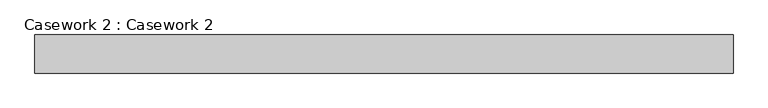
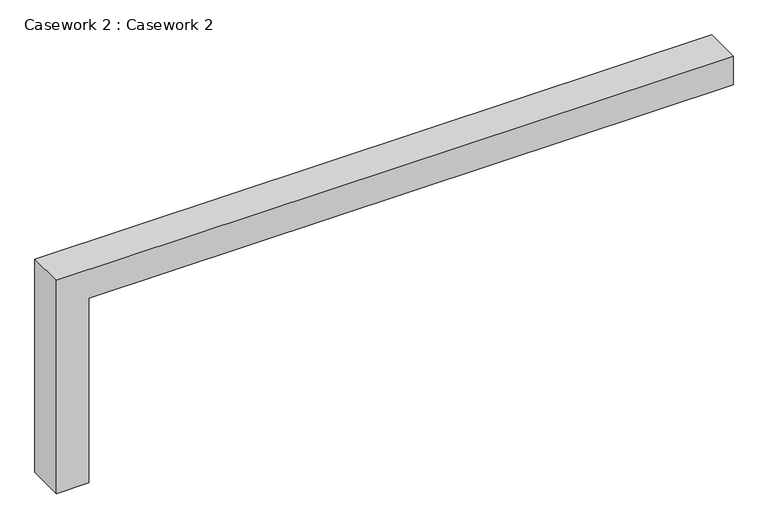
"""IFC4 building model written with IfcOpenShell, lengths in millimetres: furniture geometry, Casework 2 : Casework 2."""

from ifc_helpers import new_model, si_unit, frame, origin, place, context, project, spatial, polyline, outline, extrude, source, transform, mapped, element, save


def casework_2_casework_2_4a4ec244(model_context):
    return source(origin(), model_context, "Body", "SweptSolid", [
        extrude(outline(polyline([(5105.4, -20499.6994093), (-152.4, -20499.6994093), (-152.4, -19737.6994093), (4394.2, -19737.6994093), (4394.2, -4726.2994093), (5105.4, -4726.2994093), (5105.4, -20499.6994093)])), frame((0.0, -473.7110703, 0.0), z_axis=(0.0, 1.0, 0.0), x_axis=(0.0, 0.0, 1.0)), (0.0, 0.0, 1.0), 861.234819),
    ])


if __name__ == "__main__":
    model = new_model("IFC4")
    model_context = context("Model", 3, world=origin())
    ifc_project = project(units=[si_unit("LENGTHUNIT", "METRE", prefix="MILLI")], contexts=[model_context])
    site = spatial("IfcSite", under=ifc_project)
    building = spatial("IfcBuilding", under=site)
    placement = place(None, origin())
    casework_2_casework_2_shape = casework_2_casework_2_4a4ec244(model_context)
    element("IfcFurniture", 1, ObjectType="Casework 2 : Casework 2", at=placement, inside=building, context=model_context, shape_type="MappedRepresentation", body=[
        mapped(casework_2_casework_2_shape, transform((0.0, 0.0, 0.0), x_axis=(1.0, 0.0, 0.0), y_axis=(0.0, 1.0, 0.0), z_axis=(0.0, 0.0, 1.0))),
    ])
    save(model, "model.ifc")

# Revit data of these elements
# Element 1 (IfcFurniture, "Casework 2 : Casework 2")
#   Materials on its faces: "Clad - White"
# Materials
#   "Clad - White": class "Wood", colour RGB 242 242 238, transparency 0, Cost = 0
